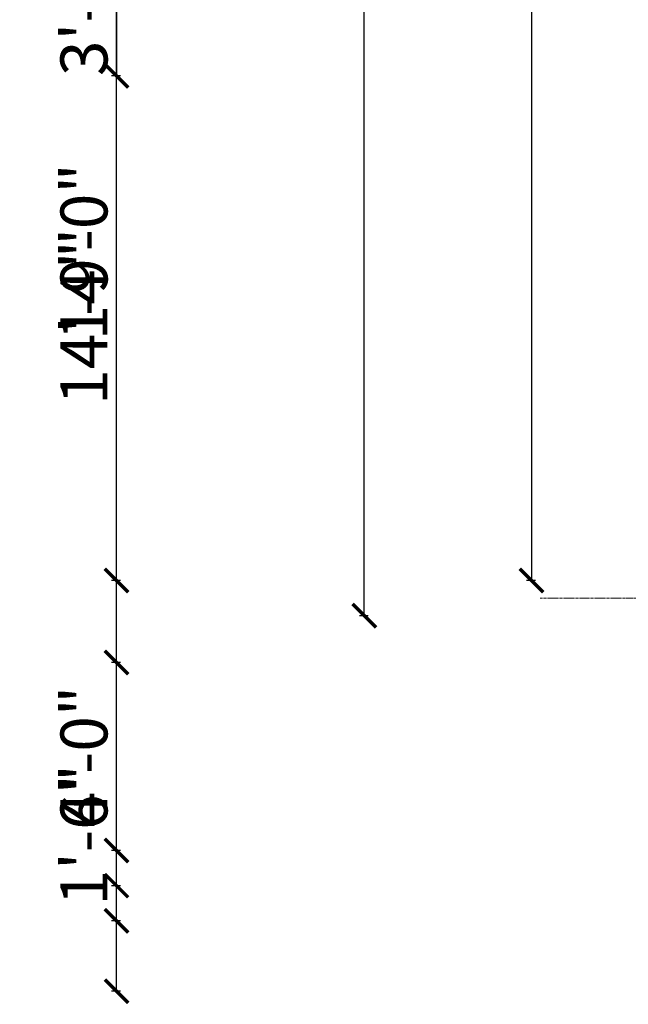
# Model space of a CAD drawing. Units: inches. Extents: x 261 to 2725, y 291 to 1454.
# Tile 1 of 35: x 261 to 417, y 409 to 661. Entities that reach past the tile are written whole.
import ezdxf

# ---------------------------------------------------------------- set-up
doc = ezdxf.new("R2010")
doc.units = ezdxf.units.IN
doc.linetypes.add('CENTER', pattern=[2, 1.25, -0.25, 0.25, -0.25])
doc.layers.add('A-ANNO-DIMS', color=136, linetype='Continuous', lineweight=18)
doc.layers.add('A-GRID', color=251, linetype='CENTER', lineweight=13)
doc.styles.get("Standard").update_dxf_attribs({"font": 'arial.ttf'})
doc.dimstyles.new('ISO-25', dxfattribs={"dimtxt": 12, "dimasz": 6, "dimexe": 1.25, "dimexo": 0.625, "dimtad": 1, "dimdec": 0, "dimlunit": 3, "dimtxsty": 'Standard', "dimblk": 'ARCHTICK', "dimcen": 2.5, "dimadec": 0, "dimazin": 0, "dimtfac": 1, "dimtdec": 0, "dimtmove": 0, "dimatfit": 3, "dimfxl": 1, "dimfxlon": 1, "dimarcsym": 0})

# ---------------------------------------------------------------- blocks, each defined once
blk = doc.blocks.new('_ArchTick')
at = {"color": 0, "linetype": 'ByBlock', "const_width": 0.15}
blk.add_lwpolyline([(-0.5, -0.5), (0.5, 0.5)], dxfattribs=at)
blk = doc.blocks.new('*D29')
at = {"layer": 'A-ANNO-DIMS', "color": 0, "lineweight": -2, "transparency": 16777216}
for p, q in [((350.37, 1231.47), (348.12, 1231.47)), ((349.37, 508.47), (349.37, 1231.47)), ((350.37, 508.47), (348.12, 508.47))]:
    blk.add_line(p, q, dxfattribs=at)
at = {"layer": 'Defpoints', "color": 0, "transparency": 16777216}
for p in [(349.37, 1231.47), (469.45, 1231.47), (469.45, 508.47)]:
    blk.add_point(p, dxfattribs=at)
at = {"layer": 'A-ANNO-DIMS', "color": 0, "lineweight": -2, "transparency": 16777216, "xscale": 6, "yscale": 6, "zscale": 6}
for p, rotation in [((349.37, 1231.47), 90), ((349.37, 508.47), 270)]:
    blk.add_blockref('_ArchTick', p, dxfattribs=dict(at, rotation=rotation))
at = {"layer": 'A-ANNO-DIMS', "color": 0, "transparency": 16777216, "insert": (342.61, 869.97), "char_height": 12, "attachment_point": 5, "rotation": 90}
blk.add_mtext('60\'-3"', dxfattribs=at)
blk = doc.blocks.new('*D30')
at = {"layer": 'A-ANNO-DIMS', "color": 0, "lineweight": -2, "transparency": 16777216}
for p, q in [((393.09, 1222.47), (390.84, 1222.47)), ((392.09, 1222.47), (392.09, 517.47)), ((393.09, 517.47), (390.84, 517.47))]:
    blk.add_line(p, q, dxfattribs=at)
at = {"layer": 'Defpoints', "color": 0, "transparency": 16777216}
for p in [(478.45, 1222.47), (392.09, 517.47), (478.45, 517.47)]:
    blk.add_point(p, dxfattribs=at)
at = {"layer": 'A-ANNO-DIMS', "color": 0, "lineweight": -2, "transparency": 16777216, "xscale": 6, "yscale": 6, "zscale": 6}
for p, rotation in [((392.09, 1222.47), 90), ((392.09, 517.47), 270)]:
    blk.add_blockref('_ArchTick', p, dxfattribs=dict(at, rotation=rotation))
at = {"layer": 'A-ANNO-DIMS', "color": 0, "transparency": 16777216, "insert": (385.34, 869.97), "char_height": 12, "attachment_point": 5, "rotation": 90}
blk.add_mtext('58\'-9"', dxfattribs=at)
blk = doc.blocks.new('*D77')
at = {"layer": 'A-ANNO-DIMS', "color": 0, "lineweight": -2, "ltscale": 0.07, "transparency": 16777216}
for p, q in [((287.06, 685.47), (284.81, 685.47)), ((286.06, 517.47), (286.06, 685.47)), ((287.06, 517.47), (284.81, 517.47))]:
    blk.add_line(p, q, dxfattribs=at)
at = {"layer": 'Defpoints', "color": 0, "ltscale": 0.07, "transparency": 16777216}
for p in [(286.06, 685.47), (478.45, 685.47), (478.45, 517.47)]:
    blk.add_point(p, dxfattribs=at)
at = {"layer": 'A-ANNO-DIMS', "color": 0, "lineweight": -2, "ltscale": 0.07, "transparency": 16777216, "xscale": 6, "yscale": 6, "zscale": 6}
for p, rotation in [((286.06, 685.47), 90), ((286.06, 517.47), 270)]:
    blk.add_blockref('_ArchTick', p, dxfattribs=dict(at, rotation=rotation))
at = {"layer": 'A-ANNO-DIMS', "color": 0, "ltscale": 0.07, "transparency": 16777216, "insert": (279.3, 601.47), "char_height": 12, "attachment_point": 5, "rotation": 90}
blk.add_mtext('14\'-0"', dxfattribs=at)
blk = doc.blocks.new('*D90')
at = {"layer": 'A-ANNO-DIMS', "color": 0, "lineweight": -2, "ltscale": 0.07, "transparency": 16777216}
for p, q in [((286.06, 430.47), (286.06, 468.49)), ((287.06, 430.47), (284.81, 430.47)), ((286.06, 412.47), (286.06, 430.47)), ((287.06, 412.47), (284.81, 412.47))]:
    blk.add_line(p, q, dxfattribs=at)
at = {"layer": 'Defpoints', "color": 0, "ltscale": 0.07, "transparency": 16777216}
for p in [(286.06, 430.47), (430.45, 430.47), (430.45, 412.47)]:
    blk.add_point(p, dxfattribs=at)
at = {"layer": 'A-ANNO-DIMS', "color": 0, "lineweight": -2, "ltscale": 0.07, "transparency": 16777216, "xscale": 6, "yscale": 6, "zscale": 6}
for p, rotation in [((286.06, 430.47), 90), ((286.06, 412.47), 270)]:
    blk.add_blockref('_ArchTick', p, dxfattribs=dict(at, rotation=rotation))
at = {"layer": 'A-ANNO-DIMS', "color": 0, "ltscale": 0.07, "transparency": 16777216, "insert": (279.3, 452.48), "char_height": 12, "attachment_point": 5, "rotation": 90}
blk.add_mtext('1\'-6"', dxfattribs=at)
blk = doc.blocks.new('*D98')
at = {"layer": 'A-ANNO-DIMS', "color": 0, "lineweight": -2, "ltscale": 0.07, "transparency": 16777216}
for p, q in [((287.06, 682.47), (284.81, 682.47)), ((286.06, 682.47), (286.06, 646.47)), ((287.06, 646.47), (284.81, 646.47))]:
    blk.add_line(p, q, dxfattribs=at)
at = {"layer": 'Defpoints', "color": 0, "ltscale": 0.07, "transparency": 16777216}
for p in [(676.45, 682.47), (286.06, 646.47), (676.45, 646.47)]:
    blk.add_point(p, dxfattribs=at)
at = {"layer": 'A-ANNO-DIMS', "color": 0, "lineweight": -2, "ltscale": 0.07, "transparency": 16777216, "xscale": 6, "yscale": 6, "zscale": 6}
for p, rotation in [((286.06, 682.47), 90), ((286.06, 646.47), 270)]:
    blk.add_blockref('_ArchTick', p, dxfattribs=dict(at, rotation=rotation))
at = {"layer": 'A-ANNO-DIMS', "color": 0, "ltscale": 0.07, "transparency": 16777216, "insert": (279.3, 664.47), "char_height": 12, "attachment_point": 5, "rotation": 90}
blk.add_mtext('3\'-0"', dxfattribs=at)
blk = doc.blocks.new('*D103')
at = {"layer": 'A-ANNO-DIMS', "color": 0, "lineweight": -2, "ltscale": 0.07, "transparency": 16777216}
for p, q in [((287.06, 1231.47), (284.81, 1231.47)), ((286.06, 439.47), (286.06, 1231.47)), ((287.06, 439.47), (284.81, 439.47))]:
    blk.add_line(p, q, dxfattribs=at)
at = {"layer": 'Defpoints', "color": 0, "ltscale": 0.07, "transparency": 16777216}
for p in [(286.06, 1231.47), (1243.08, 1231.47), (1243.08, 439.47)]:
    blk.add_point(p, dxfattribs=at)
at = {"layer": 'A-ANNO-DIMS', "color": 0, "lineweight": -2, "ltscale": 0.07, "transparency": 16777216, "xscale": 6, "yscale": 6, "zscale": 6}
for p, rotation in [((286.06, 1231.47), 90), ((286.06, 439.47), 270)]:
    blk.add_blockref('_ArchTick', p, dxfattribs=dict(at, rotation=rotation))
at = {"layer": 'A-ANNO-DIMS', "color": 0, "ltscale": 0.07, "transparency": 16777216, "insert": (279.3, 835.47), "char_height": 12, "attachment_point": 5, "rotation": 90}
blk.add_mtext('66\'-0"', dxfattribs=at)
blk = doc.blocks.new('*D106')
at = {"layer": 'A-ANNO-DIMS', "color": 0, "lineweight": -2, "ltscale": 0.07, "transparency": 16777216}
for p, q in [((287.06, 496.47), (284.81, 496.47)), ((286.06, 448.47), (286.06, 496.47)), ((287.06, 448.47), (284.81, 448.47))]:
    blk.add_line(p, q, dxfattribs=at)
at = {"layer": 'Defpoints', "color": 0, "ltscale": 0.07, "transparency": 16777216}
for p in [(286.06, 496.47), (1252.08, 496.47), (1252.08, 448.47)]:
    blk.add_point(p, dxfattribs=at)
at = {"layer": 'A-ANNO-DIMS', "color": 0, "lineweight": -2, "ltscale": 0.07, "transparency": 16777216, "xscale": 6, "yscale": 6, "zscale": 6}
for p, rotation in [((286.06, 496.47), 90), ((286.06, 448.47), 270)]:
    blk.add_blockref('_ArchTick', p, dxfattribs=dict(at, rotation=rotation))
at = {"layer": 'A-ANNO-DIMS', "color": 0, "ltscale": 0.07, "transparency": 16777216, "insert": (279.3, 472.47), "char_height": 12, "attachment_point": 5, "rotation": 90}
blk.add_mtext('4\'-0"', dxfattribs=at)
blk = doc.blocks.new('*D107')
at = {"layer": 'A-ANNO-DIMS', "color": 0, "lineweight": -2, "ltscale": 0.07, "transparency": 16777216}
for p, q in [((287.06, 673.47), (284.81, 673.47)), ((286.06, 496.47), (286.06, 673.47)), ((287.06, 496.47), (284.81, 496.47))]:
    blk.add_line(p, q, dxfattribs=at)
at = {"layer": 'Defpoints', "color": 0, "ltscale": 0.07, "transparency": 16777216}
for p in [(286.06, 673.47), (1252.08, 673.47), (1252.08, 496.47)]:
    blk.add_point(p, dxfattribs=at)
at = {"layer": 'A-ANNO-DIMS', "color": 0, "lineweight": -2, "ltscale": 0.07, "transparency": 16777216, "xscale": 6, "yscale": 6, "zscale": 6}
for p, rotation in [((286.06, 673.47), 90), ((286.06, 496.47), 270)]:
    blk.add_blockref('_ArchTick', p, dxfattribs=dict(at, rotation=rotation))
at = {"layer": 'A-ANNO-DIMS', "color": 0, "ltscale": 0.07, "transparency": 16777216, "insert": (279.3, 584.97), "char_height": 12, "attachment_point": 5, "rotation": 90}
blk.add_mtext('14\'-9"', dxfattribs=at)
blk = doc.blocks.new('*D123')
at = {"layer": 'A-ANNO-DIMS', "color": 0, "lineweight": -2, "ltscale": 0.07, "transparency": 16777216}
for p, q in [((287.06, 1054.85), (284.81, 1054.85)), ((286.06, 439.47), (286.06, 1054.85)), ((287.06, 439.47), (284.81, 439.47))]:
    blk.add_line(p, q, dxfattribs=at)
at = {"layer": 'Defpoints', "color": 0, "ltscale": 0.07, "transparency": 16777216}
for p in [(286.06, 1054.85), (2007.71, 1054.85), (2007.71, 439.47)]:
    blk.add_point(p, dxfattribs=at)
at = {"layer": 'A-ANNO-DIMS', "color": 0, "lineweight": -2, "ltscale": 0.07, "transparency": 16777216, "xscale": 6, "yscale": 6, "zscale": 6}
for p, rotation in [((286.06, 1054.85), 90), ((286.06, 439.47), 270)]:
    blk.add_blockref('_ArchTick', p, dxfattribs=dict(at, rotation=rotation))
at = {"layer": 'A-ANNO-DIMS', "color": 0, "ltscale": 0.07, "transparency": 16777216, "insert": (279.22, 747.16), "char_height": 12, "attachment_point": 5, "rotation": 90}
blk.add_mtext('51\'-3 1/2"', dxfattribs=at)

msp = doc.modelspace()

# ---------------------------------------------------------------- linework, layer by layer
at = {"layer": 'A-GRID', "ltscale": 0.5}
msp.add_line((394.31, 512.97), (1018.31, 512.97), dxfattribs=at)

# ---------------------------------------------------------------- dimensions: what is measured, and where the dimension line sits
at = {"layer": 'A-ANNO-DIMS', "ltscale": 0.07}
for base, p1, p2, picture, middle in [((286.06, 1231.47), (1243.08, 439.47), (1243.08, 1231.47), '*D103', (279.3, 835.47)), ((286.06, 1054.85), (2007.71, 439.47), (2007.71, 1054.85), '*D123', (279.22, 747.16)), ((286.06, 685.47), (478.45, 517.47), (478.45, 685.47), '*D77', (279.3, 601.47)), ((286.06, 646.47), (676.45, 682.47), (676.45, 646.47), '*D98', (279.3, 664.47)), ((286.06, 673.47), (1252.08, 496.47), (1252.08, 673.47), '*D107', (279.3, 584.97)), ((286.06, 496.47), (1252.08, 448.47), (1252.08, 496.47), '*D106', (279.3, 472.47)), ((286.06, 430.47), (430.45, 412.47), (430.45, 430.47), '*D90', (279.3, 452.48))]:
    dim = msp.add_linear_dim(base=base, p1=p1, p2=p2, angle=90, dimstyle='ISO-25', override={"dimdec": 1, "dimlfac": 1, "dimrnd": 0, "dimzin": 1, "dimdsep": 46, "dimlunit": 4, "dimfrac": 2}, dxfattribs=at)
    dim.commit()
    dim.dimension.update_dxf_attribs({"geometry": picture, "text_midpoint": middle})
at = {"layer": 'A-ANNO-DIMS'}
for base, p1, p2, picture, middle in [((349.37, 1231.47), (469.45, 508.47), (469.45, 1231.47), '*D29', (342.61, 869.97)), ((392.09, 517.47), (478.45, 1222.47), (478.45, 517.47), '*D30', (385.34, 869.97))]:
    dim = msp.add_linear_dim(base=base, p1=p1, p2=p2, angle=90, dimstyle='ISO-25', override={"dimclrd": 0, "dimclre": 0, "dimclrt": 0}, dxfattribs=at)
    dim.commit()
    dim.dimension.update_dxf_attribs({"geometry": picture, "text_midpoint": middle})

doc.saveas('drawing.dxf')
